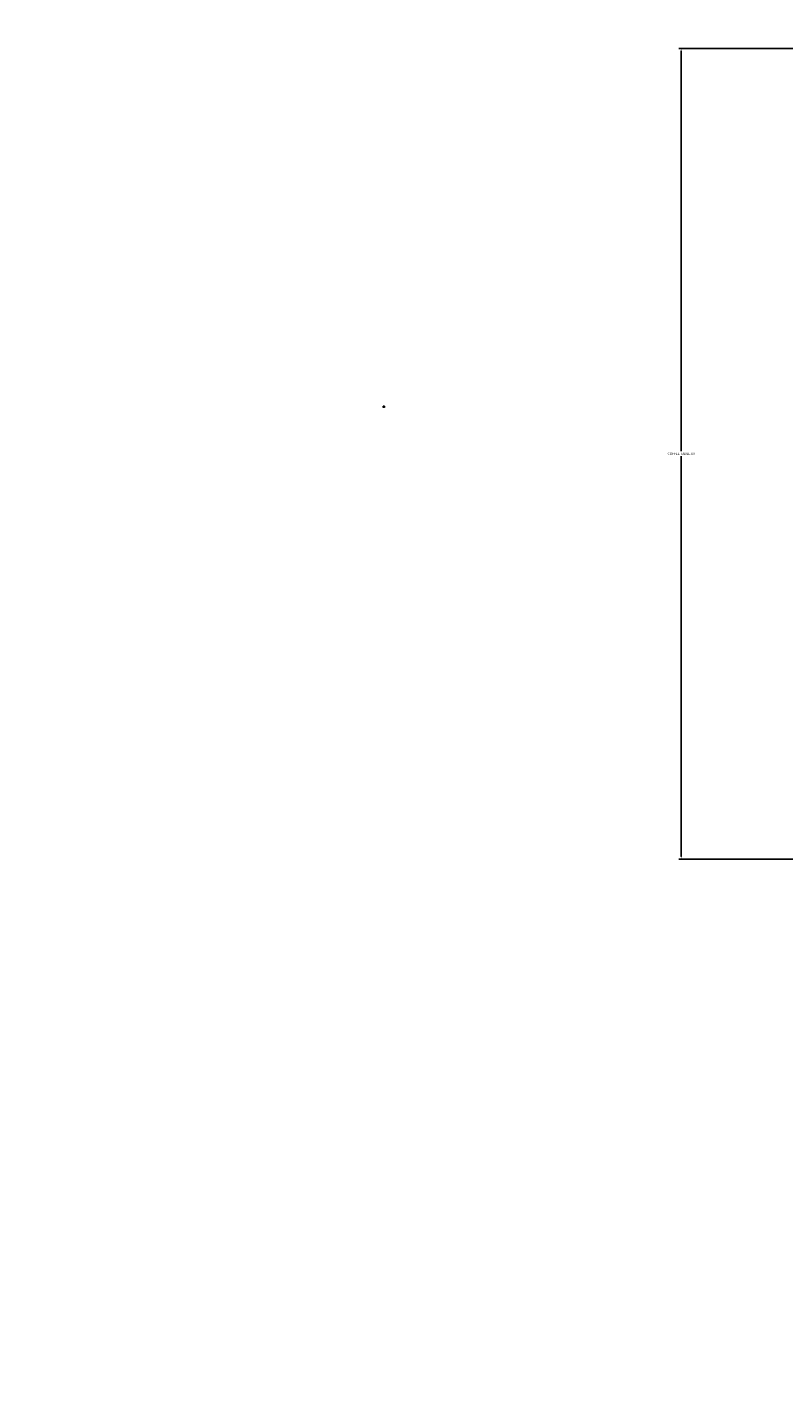
# Model space of a CAD drawing. Units: inches. Extents: x 2549 to 3108, y 1683 to 2362.
# Tile 22 of 30: x 2893 to 2949, y 1979 to 2080. Entities that reach past the tile are written whole.
import ezdxf

# ---------------------------------------------------------------- set-up
doc = ezdxf.new("R2010")
doc.units = ezdxf.units.IN
doc.layers.add('A-ANNO-DIMS', color=2, linetype='Continuous', lineweight=18)
doc.layers.add('C-PKNG-VEHI-PATT', color=251, linetype='Continuous', lineweight=13, true_color=0x636466)
doc.layers.add('C-PVMT-PATT', color=9, linetype='Continuous', lineweight=13, true_color=0xc7c8ca)
doc.styles.get("Standard").update_dxf_attribs({"font": 'arial.ttf'})
doc.dimstyles.get("Standard").update_dxf_attribs({"dimtxt": 0.18, "dimasz": 0.18, "dimexe": 0.18, "dimexo": 0.0625, "dimgap": 0.09, "dimtad": 0, "dimtih": 1, "dimtoh": 1, "dimdec": 4, "dimzin": 0, "dimdsep": 46, "dimtxsty": 'Standard', "dimcen": 0.09, "dimadec": 0, "dimazin": 0, "dimtfac": 1, "dimtdec": 4, "dimtofl": 0, "dimtmove": 0, "dimatfit": 3, "dimfxl": 1, "dimtolj": 1, "dimtzin": 0, "dimarcsym": 0})

# ---------------------------------------------------------------- blocks, each defined once
blk = doc.blocks.new('*D22')
at = {"layer": 'A-ANNO-DIMS', "color": 0, "lineweight": -2, "transparency": 16777216}
for p, q in [((2950.03, 2078.61), (2940.91, 2078.61)), ((2941.09, 2078.43), (2941.09, 2048.8)), ((2941.09, 2018.79), (2941.09, 2048.43)), ((2950.03, 2018.61), (2940.91, 2018.61))]:
    blk.add_line(p, q, dxfattribs=at)
at = {"layer": 'A-ANNO-DIMS', "color": 0, "transparency": 16777216}
for points in [[(2941.06, 2078.43), (2941.12, 2078.43), (2941.09, 2078.61)], [(2941.06, 2018.79), (2941.12, 2018.79), (2941.09, 2018.61)]]:
    blk.add_solid(points, dxfattribs=at)
at = {"layer": 'Defpoints', "color": 0, "transparency": 16777216}
for p in [(2950.09, 2078.61), (2941.09, 2018.61), (2950.09, 2018.61)]:
    blk.add_point(p, dxfattribs=at)
at = {"layer": 'A-ANNO-DIMS', "color": 0, "transparency": 16777216, "insert": (2941.09, 2048.61), "char_height": 0.18, "attachment_point": 5}
blk.add_mtext('\\A1;COFFEE TABLE 60', dxfattribs=at)
blk = doc.blocks.new('*D46')
at = {"layer": 'A-ANNO-DIMS', "color": 0, "lineweight": -2, "transparency": 16777216}
for p, q in [((2812.64, 2140.46), (2812.64, 1683.44)), ((3034.64, 2134.46), (3034.64, 1683.44)), ((2812.82, 1683.62), (2923.35, 1683.62)), ((3034.46, 1683.62), (2923.93, 1683.62))]:
    blk.add_line(p, q, dxfattribs=at)
at = {"layer": 'A-ANNO-DIMS', "color": 0, "transparency": 16777216}
for points in [[(2812.82, 1683.65), (2812.82, 1683.59), (2812.64, 1683.62)], [(3034.46, 1683.65), (3034.46, 1683.59), (3034.64, 1683.62)]]:
    blk.add_solid(points, dxfattribs=at)
at = {"layer": 'Defpoints', "color": 0, "transparency": 16777216}
for p in [(2812.64, 2140.52), (3034.64, 2134.52), (3034.64, 1683.62)]:
    blk.add_point(p, dxfattribs=at)
at = {"layer": 'A-ANNO-DIMS', "color": 0, "transparency": 16777216, "insert": (2923.64, 1683.62), "char_height": 0.18, "attachment_point": 5}
blk.add_mtext('\\A1;222', dxfattribs=at)
blk = doc.blocks.new('*D64')
at = {"layer": 'A-ANNO-DIMS', "color": 0, "lineweight": -2, "transparency": 16777216}
for p, q in [((2919.01, 2052.09), (2919.19, 2052.09)), ((2919.1, 2052), (2919.1, 2052.18)), ((3101.9, 2052.09), (3033.53, 2052.09))]:
    blk.add_line(p, q, dxfattribs=at)
at = {"layer": 'A-ANNO-DIMS', "color": 0, "transparency": 16777216}
blk.add_solid([(3033.53, 2052.12), (3033.53, 2052.06), (3033.35, 2052.09)], dxfattribs=at)
at = {"layer": 'Defpoints', "color": 0, "transparency": 16777216}
for p in [(2919.1, 2052.09), (3033.35, 2052.09)]:
    blk.add_point(p, dxfattribs=at)
at = {"layer": 'A-ANNO-DIMS', "color": 0, "transparency": 16777216, "insert": (3102.64, 2052.09), "char_height": 0.18, "attachment_point": 5}
blk.add_mtext('\\A1;2X R114.25', dxfattribs=at)

msp = doc.modelspace()

# ---------------------------------------------------------------- hatches: boundary and pattern name
at = {"layer": 'C-PKNG-VEHI-PATT'}
h = msp.add_hatch(color=256, dxfattribs=at)
h.dxf.hatch_style = 1
edge = h.paths.add_edge_path()
edge.add_ellipse((2935.7258, 1791.964), major_axis=(-50.66, 0), ratio=0.84230387, start_angle=248.165046, end_angle=265.722579)
edge.add_line((2938.911, 1834.5507), (2925.8653, 1834.5507))
edge.add_ellipse((2929.0505, 1791.964), major_axis=(50.66, 0), ratio=0.84230387, start_angle=94.277421, end_angle=111.834954)
edge.add_line((2912.8508, 1832.3947), (2914.2044, 1822.2495))
edge.add_ellipse((2930.6538, 1783.1023), major_axis=(-49.3014, 0), ratio=0.84230387, start_angle=-85.12993, end_angle=-67.208085, ccw=False)
edge.add_line((2927.1247, 1824.5225), (2937.6516, 1824.5225))
edge.add_ellipse((2934.1225, 1783.1023), major_axis=(49.3014, 0), ratio=0.84230387, start_angle=67.208085, end_angle=85.12993, ccw=False)
edge.add_line((2950.5719, 1822.2495), (2951.9255, 1832.3947))
edge = h.paths.add_edge_path()
edge.add_ellipse((2903.4793, 1857.3351), major_axis=(-34.7979, 0), ratio=0.84230387, start_angle=180, end_angle=209.43857)
edge.add_ellipse((2961.297, 1857.3351), major_axis=(34.7979, 0), ratio=0.84230387, start_angle=150.56143, end_angle=180)
edge.add_line((2926.4991, 1857.3351), (2926.4991, 1843.7609))
edge.add_ellipse((2924.1251, 1844.3143), major_axis=(-0.2209, 3.9278), ratio=0.60383358, start_angle=89.002014, end_angle=253.657408, ccw=False)
edge.add_line((2921.7512, 1844.2222), (2921.7512, 1853.3975))
edge.add_line((2921.7512, 1853.3975), (2925.269, 1855.8484))
edge.add_ellipse((2925.4782, 1855.4931), major_axis=(0.4584, 0), ratio=0.84230387, start_angle=90, end_angle=134.480211, ccw=False)
edge.add_line((2925.4782, 1855.8792), (2926.4991, 1855.8792))
edge.add_line((2926.4991, 1855.8792), (2926.4991, 1857.3351))
edge.add_ellipse((2961.297, 1857.3351), major_axis=(34.7979, 0), ratio=0.84230387, start_angle=150.56143, end_angle=180, ccw=False)
edge.add_line((2932.3882, 1873.6501), (2932.3882, 1875.7801))
edge.add_ellipse((2932.3882, 1875.3939), major_axis=(0.4584, 0), ratio=0.84230387, start_angle=90, end_angle=127.93313)
edge.add_line((2932.1366, 1875.7167), (2928.5915, 1873.7564))
edge.add_ellipse((2899.9271, 2002.4692), major_axis=(155.4756, 0), ratio=0.84230387, start_angle=-80.743434, end_angle=-77.445067, ccw=False)
edge.add_ellipse((2949.4402, 1715.2151), major_axis=(-189.1422, 0), ratio=0.84230387, start_angle=-79.790461, end_angle=-77.555373)
edge.add_ellipse((3300.3614, 1852.5642), major_axis=(-386.1662, 0), ratio=0.84230387, start_angle=-2.863715, end_angle=2.198541)
edge.add_ellipse((2929.0505, 1792.5159), major_axis=(-55.6192, 0), ratio=0.84230387, start_angle=-85.917589, end_angle=-72.280047, ccw=False)
edge.add_line((2925.7129, 1839.2798), (2939.0634, 1839.2798))
edge.add_ellipse((2935.7258, 1792.5159), major_axis=(55.6192, 0), ratio=0.84230387, start_angle=72.280047, end_angle=85.917589, ccw=False)
edge.add_ellipse((2564.4149, 1852.5642), major_axis=(-386.1662, 0), ratio=0.84230387, start_angle=177.801459, end_angle=182.863715)
edge.add_ellipse((2915.3361, 1715.2151), major_axis=(189.1422, 0), ratio=0.84230387, start_angle=77.555373, end_angle=79.790461)
edge.add_ellipse((2964.8492, 2002.4692), major_axis=(-155.4756, 0), ratio=0.84230387, start_angle=77.445067, end_angle=80.743434, ccw=False)
edge.add_line((2936.1848, 1873.7564), (2932.6397, 1875.7167))
edge.add_ellipse((2932.3882, 1875.3939), major_axis=(0.4584, 0), ratio=0.84230387, start_angle=52.06687, end_angle=90)
edge.add_line((2932.3882, 1875.7801), (2932.3882, 1873.6501))
edge.add_ellipse((2903.4793, 1857.3351), major_axis=(-34.7979, 0), ratio=0.84230387, start_angle=180, end_angle=209.43857, ccw=False)
edge.add_line((2938.2772, 1857.3351), (2938.2772, 1855.8792))
edge.add_line((2938.2772, 1855.8792), (2939.4059, 1855.8792))
edge.add_ellipse((2939.2981, 1855.4931), major_axis=(-0.4584, 0), ratio=0.84230387, start_angle=225.519789, end_angle=270, ccw=False)
edge.add_line((2939.5903, 1855.7906), (2943.0251, 1853.3975))
edge.add_line((2943.0251, 1853.3975), (2943.0251, 1844.2222))
edge.add_ellipse((2940.6512, 1844.3143), major_axis=(0.2209, 3.9278), ratio=0.60383358, start_angle=106.342592, end_angle=270.997986, ccw=False)
edge.add_line((2938.2772, 1843.7609), (2938.2772, 1857.3351))
edge = h.paths.add_edge_path()
edge.add_ellipse((2932.3882, 1865.1973), major_axis=(91.081, 0), ratio=0.84230387, start_angle=256.401865, end_angle=283.598135, ccw=False)
edge.add_line((2914.2044, 1790.0239), (2914.2044, 1778.3622))
edge.add_ellipse((2932.3882, 1853.5356), major_axis=(91.081, 0), ratio=0.84230387, start_angle=256.401865, end_angle=283.598135)
edge.add_line((2950.5719, 1778.3622), (2950.5719, 1790.0239))
edge = h.paths.add_edge_path()
edge.add_ellipse((2948.7383, 1772.3145), major_axis=(1.8336, 0), ratio=0.84230387, start_angle=0, end_angle=90)
edge.add_line((2948.7383, 1773.859), (2916.038, 1773.859))
edge.add_ellipse((2916.038, 1772.3145), major_axis=(1.8336, 0), ratio=0.84230387, start_angle=90, end_angle=180)
edge.add_line((2914.2044, 1772.3145), (2914.2044, 1760.2558))
edge.add_line((2914.2044, 1760.2558), (2950.5719, 1760.2558))
edge.add_line((2950.5719, 1760.2558), (2950.5719, 1772.3145))
h.paths.add_polyline_path([(2748.8496, 2101.6383), (2798.148, 2101.6383), (2798.148, 2111.4248), (2748.8496, 2111.4248)], flags=9)
h.paths.add_polyline_path([(2685.2081, 2101.489), (2719.3253, 2101.489), (2719.3253, 2111.2819), (2685.2081, 2111.2819)], flags=9)
h.paths.add_polyline_path([(2814.6852, 1907.1328), (2847.8384, 1907.1328), (2847.8384, 1916.9258), (2814.6852, 1916.9258)], flags=9)
h.paths.add_polyline_path([(2814.3906, 1835.5864), (2848.0172, 1835.5864), (2848.0172, 1845.3794), (2814.3906, 1845.3794)], flags=9)
h.paths.add_polyline_path([(2800.5245, 1759.1674), (2853.7435, 1759.1674), (2853.7435, 1768.954), (2800.5245, 1768.954)], flags=9)
h.paths.add_polyline_path([(2972.4611, 1807.3305), (3015.3943, 1807.3305), (3015.3943, 1817.117), (2972.4611, 1817.117)], flags=9)
h.paths.add_polyline_path([(2902.3327, 1888.6731), (2937.9131, 1888.6731), (2937.9131, 1898.4661), (2902.3327, 1898.4661)], flags=9)
h.paths.add_polyline_path([(2712.1779, 1878.9039), (2754.1257, 1878.9039), (2754.1257, 1888.6904), (2712.1779, 1888.6904)], flags=9)
h.paths.add_polyline_path([(2614.0056, 2012.812), (2650.0251, 2012.812), (2650.0251, 2022.4371), (2614.0056, 2022.4371)], flags=9)
h.paths.add_polyline_path([(2713.3129, 2003.1645), (2747.4237, 2003.1645), (2747.4237, 2012.951), (2713.3129, 2012.951)], flags=9)
h.paths.add_polyline_path([(2950.1379, 2001.6934), (2982.2992, 2001.6934), (2982.2992, 2011.48), (2950.1379, 2011.48)], flags=9)
h.paths.add_polyline_path([(2940.864, 2238.5537), (2997.5066, 2238.5537), (2997.5066, 2248.3466), (2940.864, 2248.3466)], flags=9)
h.paths.add_polyline_path([(2821.5457, 2202.8348), (2855.663, 2202.8348), (2855.663, 2212.6278), (2821.5457, 2212.6278)], flags=9)
h.paths.add_polyline_path([(2661.8026, 2238.6249), (2718.4451, 2238.6249), (2718.4451, 2248.4179), (2661.8026, 2248.4179)], flags=9)
at = {"layer": 'C-PVMT-PATT'}
h = msp.add_hatch(color=256, dxfattribs=at)
h.dxf.hatch_style = 1
h.paths.add_polyline_path([(3067.6427, 2305.5237), (2605.6427, 2305.5237), (2605.6427, 2074.5237), (2629.6427, 2074.5237), (2629.6427, 2281.5237), (3043.6427, 2281.5237), (3043.6427, 1885.5237), (3043.6427, 1872.8745), (3031.1672, 1872.8745), (3031.1672, 1862.5731), (2995.8054, 1862.5731), (2995.8054, 1872.8745), (2983.1752, 1872.8745), (2983.1752, 1885.5237), (2881.6427, 1885.5237), (2881.6427, 1795.5237), (2751.0977, 1795.5237), (2751.0977, 1761.5237), (2786.1577, 1761.5237), (2786.1577, 1723.5237), (2881.84, 1723.5237), (2881.84, 1714.5237), (3067.6427, 1714.5237), (3067.6427, 1723.5237)])
edge = h.paths.add_edge_path(flags=16)
edge.add_ellipse((2949.4402, 1710.9683), major_axis=(-194.1014, 0), ratio=0.84230387, start_angle=-77.874034, end_angle=-76.219471, ccw=False)
edge.add_ellipse((2949.4402, 1715.2151), major_axis=(-189.1422, 0), ratio=0.84230387, start_angle=-79.790461, end_angle=-77.555373, ccw=False)
edge.add_ellipse((2899.9271, 2002.4692), major_axis=(155.4756, 0), ratio=0.84230387, start_angle=-80.743434, end_angle=-77.445067)
edge.add_line((2928.5915, 1873.7564), (2932.3882, 1875.8558))
edge.add_line((2932.3882, 1875.8558), (2936.1848, 1873.7564))
edge.add_ellipse((2964.8492, 2002.4692), major_axis=(-155.4756, 0), ratio=0.84230387, start_angle=77.445067, end_angle=80.743434)
edge.add_ellipse((2915.3361, 1715.2151), major_axis=(189.1422, 0), ratio=0.84230387, start_angle=77.555373, end_angle=79.790461, ccw=False)
edge.add_ellipse((2915.3361, 1710.9683), major_axis=(-194.1014, 0), ratio=0.84230387, start_angle=256.219471, end_angle=257.874034, ccw=False)
edge.add_ellipse((2628.2871, 1850.2612), major_axis=(-327.2532, 0), ratio=0.84230387, start_angle=182.17995, end_angle=183.650428, ccw=False)
edge.add_ellipse((2955.5637, 1861.9334), major_axis=(-0.9168, 0), ratio=0.84230387, start_angle=180, end_angle=270, ccw=False)
edge.add_line((2956.4805, 1862.3857), (2956.4805, 1846.4866))
edge.add_ellipse((2955.5637, 1846.939), major_axis=(-0.9168, 0), ratio=0.84230387, start_angle=90, end_angle=180, ccw=False)
edge.add_ellipse((-3607.0606, 1835.832), major_axis=(-6562.6242, 0), ratio=0.84230387, start_angle=179.61613322, end_angle=180.09022909, ccw=False)
edge.add_ellipse((2955.5637, 1791.0926), major_axis=(0.9168, 0), ratio=0.84230387, start_angle=0, end_angle=90, ccw=False)
edge.add_line((2956.4805, 1791.545), (2956.4805, 1775.6459))
edge.add_ellipse((2955.5637, 1776.0982), major_axis=(0.9168, 0), ratio=0.84230387, start_angle=270, end_angle=360, ccw=False)
edge.add_ellipse((-3607.0606, 1835.832), major_axis=(-6562.6242, 0), ratio=0.84230387, start_angle=179.3813568, end_angle=179.47172853, ccw=False)
edge.add_ellipse((2954.5907, 1763.8768), major_axis=(-1.3752, 0), ratio=0.84230387, start_angle=179.371763, end_angle=248.464757, ccw=False)
edge.add_ellipse((-3607.519, 1835.832), major_axis=(-6564.0409, 0), ratio=0.842303863, start_angle=179.35344594, end_angle=179.37176282, ccw=False)
edge.add_ellipse((2952.6829, 1761.8002), major_axis=(3.2503, 0), ratio=0.84230387, start_angle=-90, end_angle=-0.646554, ccw=False)
edge.add_line((2952.6829, 1759.0625), (2912.0934, 1759.0625))
edge.add_ellipse((2912.0934, 1761.8002), major_axis=(3.2503, 0), ratio=0.84230387, start_angle=180.646554, end_angle=270, ccw=False)
edge.add_ellipse((9472.2953, 1835.832), major_axis=(-6564.0409, 0), ratio=0.842303871, start_angle=0.62823722, end_angle=0.6465541, ccw=False)
edge.add_ellipse((2910.1856, 1763.8768), major_axis=(1.3752, 0), ratio=0.84230387, start_angle=111.535244, end_angle=180.628237, ccw=False)
edge.add_ellipse((9471.8369, 1835.832), major_axis=(-6562.6242, 0), ratio=0.84230387, start_angle=0.52827147, end_angle=0.6465541, ccw=False)
edge.add_ellipse((2909.2126, 1776.0982), major_axis=(-0.9168, 0), ratio=0.84230387, start_angle=0, end_angle=90, ccw=False)
edge.add_line((2908.2958, 1775.6459), (2908.2958, 1791.545))
edge.add_ellipse((2909.2126, 1791.0926), major_axis=(-0.9168, 0), ratio=0.84230387, start_angle=-90, end_angle=0, ccw=False)
edge.add_ellipse((9471.8369, 1835.832), major_axis=(-6562.6242, 0), ratio=0.84230387, start_angle=-0.09022909, end_angle=0.38386678, ccw=False)
edge.add_ellipse((2909.2126, 1846.939), major_axis=(-0.9168, 0), ratio=0.84230387, start_angle=0, end_angle=90, ccw=False)
edge.add_line((2908.2958, 1846.4866), (2908.2958, 1862.3857))
edge.add_ellipse((2909.2126, 1861.9334), major_axis=(0.9168, 0), ratio=0.84230387, start_angle=90, end_angle=180, ccw=False)
edge.add_ellipse((3236.4892, 1850.2612), major_axis=(327.2532, 0), ratio=0.84230387, start_angle=176.349572, end_angle=177.82005, ccw=False)
edge = h.paths.add_edge_path(flags=0)
edge.add_ellipse((2903.4793, 1857.3351), major_axis=(-34.7979, 0), ratio=0.84230387, start_angle=180, end_angle=209.43857, ccw=False)
edge.add_line((2938.2772, 1857.3351), (2938.2772, 1855.8792))
edge.add_line((2938.2772, 1855.8792), (2939.4631, 1855.8792))
edge.add_line((2939.4631, 1855.8792), (2943.0251, 1853.3975))
edge.add_line((2943.0251, 1853.3975), (2943.0251, 1844.2222))
edge.add_ellipse((2940.6512, 1844.3143), major_axis=(0.2209, 3.9278), ratio=0.60383358, start_angle=106.342592, end_angle=270.997986, ccw=False)
edge.add_line((2938.2772, 1843.7609), (2938.2772, 1857.3351))
edge.add_ellipse((2903.4793, 1857.3351), major_axis=(-34.7979, 0), ratio=0.84230387, start_angle=180, end_angle=209.43857)
edge.add_ellipse((2961.297, 1857.3351), major_axis=(34.7979, 0), ratio=0.84230387, start_angle=150.56143, end_angle=180)
edge.add_line((2926.4991, 1857.3351), (2926.4991, 1843.7609))
edge.add_ellipse((2924.1251, 1844.3143), major_axis=(-0.2209, 3.9278), ratio=0.60383358, start_angle=89.002014, end_angle=253.657408, ccw=False)
edge.add_line((2921.7512, 1844.2222), (2921.7512, 1853.3975))
edge.add_line((2921.7512, 1853.3975), (2925.3132, 1855.8792))
edge.add_line((2925.3132, 1855.8792), (2926.4991, 1855.8792))
edge.add_line((2926.4991, 1855.8792), (2926.4991, 1857.3351))
edge.add_ellipse((2961.297, 1857.3351), major_axis=(34.7979, 0), ratio=0.84230387, start_angle=150.56143, end_angle=180, ccw=False)
edge = h.paths.add_edge_path(flags=0)
edge.add_ellipse((2929.0505, 1791.964), major_axis=(50.66, 0), ratio=0.84230387, start_angle=94.277421, end_angle=111.834954, ccw=False)
edge.add_line((2925.8653, 1834.5507), (2938.911, 1834.5507))
edge.add_ellipse((2935.7258, 1791.964), major_axis=(-50.66, 0), ratio=0.84230387, start_angle=248.165046, end_angle=265.722579, ccw=False)
edge.add_line((2951.9255, 1832.3947), (2950.5719, 1822.2495))
edge.add_ellipse((2934.1225, 1783.1023), major_axis=(49.3014, 0), ratio=0.84230387, start_angle=67.208085, end_angle=85.12993)
edge.add_line((2937.6516, 1824.5225), (2927.1247, 1824.5225))
edge.add_ellipse((2930.6538, 1783.1023), major_axis=(-49.3014, 0), ratio=0.84230387, start_angle=-85.12993, end_angle=-67.208085)
edge.add_line((2914.2044, 1822.2495), (2912.8508, 1832.3947))
edge = h.paths.add_edge_path(flags=0)
edge.add_line((2910.1338, 1829.4651), (2912.6432, 1821.2711))
edge.add_ellipse((5203.7787, 1816.4367), major_axis=(-2291.1426, 0), ratio=0.84230387, start_angle=-0.1208974, end_angle=0.3640763)
edge.add_line((2912.7012, 1801.8782), (2910.3305, 1792.5698))
edge.add_ellipse((9471.8369, 1835.832), major_axis=(-6561.7074, 0), ratio=0.84230387, start_angle=0.05559431, end_angle=0.37776419, ccw=False)
edge = h.paths.add_edge_path(flags=0)
edge.add_ellipse((-3607.0606, 1835.832), major_axis=(6561.7074, 0), ratio=0.84230387, start_angle=-0.37776419, end_angle=-0.05559431, ccw=False)
edge.add_line((2954.4458, 1792.5698), (2952.0751, 1801.8782))
edge.add_ellipse((660.9976, 1816.4367), major_axis=(2291.1426, 0), ratio=0.84230387, start_angle=-0.3640763, end_angle=0.1208974)
edge.add_line((2952.1331, 1821.2711), (2954.6425, 1829.4651))
edge = h.paths.add_edge_path(flags=0)
edge.add_ellipse((2932.3882, 1865.1973), major_axis=(91.081, 0), ratio=0.84230387, start_angle=256.401865, end_angle=283.598135)
edge.add_line((2950.5719, 1790.0239), (2950.5719, 1778.3622))
edge.add_ellipse((2932.3882, 1853.5356), major_axis=(91.081, 0), ratio=0.84230387, start_angle=256.401865, end_angle=283.598135, ccw=False)
edge.add_line((2914.2044, 1778.3622), (2914.2044, 1790.0239))
edge = h.paths.add_edge_path(flags=0)
edge.add_line((2916.038, 1773.859), (2948.7383, 1773.859))
edge.add_ellipse((2948.7383, 1772.3145), major_axis=(1.8336, 0), ratio=0.84230387, start_angle=0, end_angle=90, ccw=False)
edge.add_line((2950.5719, 1772.3145), (2950.5719, 1760.2558))
edge.add_line((2950.5719, 1760.2558), (2914.2044, 1760.2558))
edge.add_line((2914.2044, 1760.2558), (2914.2044, 1772.3145))
edge.add_ellipse((2916.038, 1772.3145), major_axis=(1.8336, 0), ratio=0.84230387, start_angle=90, end_angle=180, ccw=False)
h.paths.add_polyline_path([(2629.6427, 1978.5237), (2605.6427, 1978.5237), (2605.6427, 1723.5237), (2629.6427, 1723.5237), (2629.6427, 1795.5237)], flags=17)
h.paths.add_polyline_path([(2800.5245, 1759.1674), (2853.7435, 1759.1674), (2853.7435, 1768.954), (2800.5245, 1768.954)], flags=24)
h.paths.add_polyline_path([(2972.4611, 1807.3305), (3015.3943, 1807.3305), (3015.3943, 1817.117), (2972.4611, 1817.117)], flags=24)

# ---------------------------------------------------------------- dimensions: what is measured, and where the dimension line sits
at = {"layer": 'A-ANNO-DIMS'}
dim = msp.add_linear_dim(base=(3034.6427, 1683.6237), p1=(2812.6427, 2140.5237), p2=(3034.6427, 2134.5237), dimstyle='Standard', override={"dimdec": 0, "dimlfac": 1, "dimrnd": 0, "dimzin": 0, "dimdsep": 46, "dimlunit": 2}, dxfattribs=at)
dim.commit()
dim.dimension.update_dxf_attribs({"geometry": '*D46', "text_midpoint": (2923.6427, 1683.6237)})
dim = msp.add_linear_dim(base=(2941.0931, 2018.6146), p1=(2950.0931, 2078.6146), p2=(2950.0931, 2018.6146), angle=270, text='COFFEE TABLE <>', dimstyle='Standard', override={"dimdec": 0, "dimlfac": 1, "dimrnd": 0, "dimzin": 0, "dimdsep": 46, "dimlunit": 2}, dxfattribs=at)
dim.commit()
dim.dimension.update_dxf_attribs({"geometry": '*D22', "text_midpoint": (2941.0931, 2048.6146)})
dim = msp.add_radius_dim(center=(2919.097, 2052.0905), mpoint=(3033.347, 2052.091), text='2X <>', dimstyle='Standard', override={"dimdec": 2, "dimlfac": 1, "dimrnd": 0, "dimzin": 0, "dimdsep": 46, "dimlunit": 2}, dxfattribs=at)
dim.commit()
dim.dimension.update_dxf_attribs({"geometry": '*D64', "text_midpoint": (3101.897, 2052.0913), "dimtype": 164})

doc.saveas('drawing.dxf')
